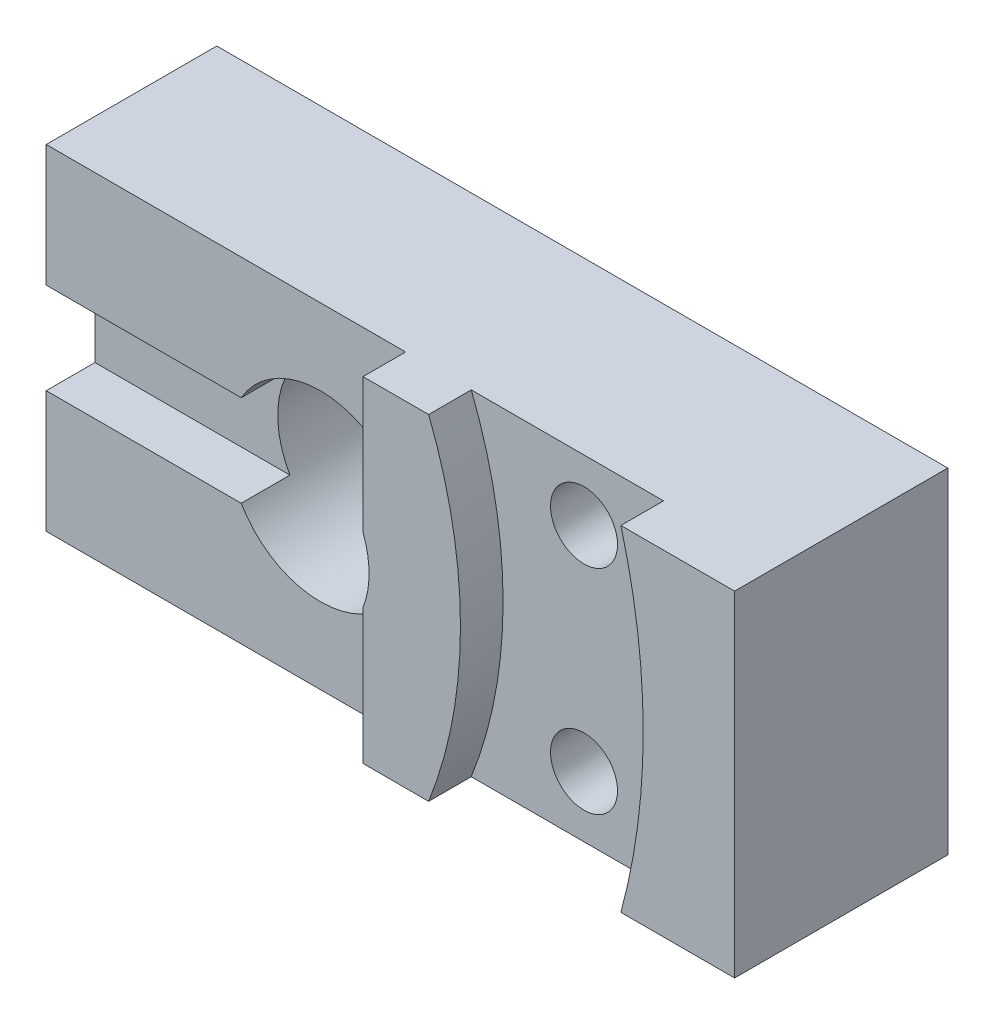
ISO-10303-21;
HEADER;
FILE_DESCRIPTION(('STEP AP214'),'2;1');
FILE_NAME('part.step','',(''),(''),'','','');
FILE_SCHEMA(('AUTOMOTIVE_DESIGN { 1 0 10303 214 1 1 1 1 }'));
ENDSEC;
DATA;
#1=APPLICATION_CONTEXT('core data for automotive mechanical design processes');
#2=APPLICATION_PROTOCOL_DEFINITION('international standard','automotive_design',2000,#1);
#3=PRODUCT_CONTEXT('',#1,'mechanical');
#4=PRODUCT('Part','Part','',(#3));
#5=PRODUCT_RELATED_PRODUCT_CATEGORY('part','',(#4));
#6=PRODUCT_DEFINITION_FORMATION('','',#4);
#7=PRODUCT_DEFINITION_CONTEXT('part definition',#1,'design');
#8=PRODUCT_DEFINITION('design','',#6,#7);
#9=PRODUCT_DEFINITION_SHAPE('','',#8);
#10=(LENGTH_UNIT() NAMED_UNIT(*) SI_UNIT(.MILLI.,.METRE.));
#11=(NAMED_UNIT(*) PLANE_ANGLE_UNIT() SI_UNIT($,.RADIAN.));
#12=(NAMED_UNIT(*) SI_UNIT($,.STERADIAN.) SOLID_ANGLE_UNIT());
#13=UNCERTAINTY_MEASURE_WITH_UNIT(LENGTH_MEASURE(1.E-05),#10,'distance_accuracy_value','');
#14=(GEOMETRIC_REPRESENTATION_CONTEXT(3) GLOBAL_UNCERTAINTY_ASSIGNED_CONTEXT((#13)) GLOBAL_UNIT_ASSIGNED_CONTEXT((#10,
#11,#12)) REPRESENTATION_CONTEXT('',''));
#15=CARTESIAN_POINT('',(0.,0.,0.));
#16=DIRECTION('',(0.,0.,1.));
#17=DIRECTION('',(1.,0.,0.));
#18=AXIS2_PLACEMENT_3D('',#15,#16,#17);
#19=CARTESIAN_POINT('',(0.,0.,28.));
#20=DIRECTION('',(0.,0.,-1.));
#21=DIRECTION('',(-1.,0.,0.));
#22=AXIS2_PLACEMENT_3D('',#19,#20,#21);
#23=PLANE('',#22);
#24=DIRECTION('',(0.,1.,0.));
#25=VECTOR('',#24,1.);
#26=CARTESIAN_POINT('',(-1.,0.,28.));
#27=LINE('',#26,#25);
#28=CARTESIAN_POINT('',(-1.,0.,28.));
#29=VERTEX_POINT('',#28);
#30=CARTESIAN_POINT('',(-1.,20.,28.));
#31=VERTEX_POINT('',#30);
#32=EDGE_CURVE('E204',#29,#31,#27,.T.);
#33=ORIENTED_EDGE('',*,*,#32,.T.);
#34=DIRECTION('',(-1.,0.,0.));
#35=VECTOR('',#34,1.);
#36=CARTESIAN_POINT('',(-1.,20.,28.));
#37=LINE('',#36,#35);
#38=CARTESIAN_POINT('',(-2.00961894323342,20.,28.));
#39=VERTEX_POINT('',#38);
#40=EDGE_CURVE('E328',#31,#39,#37,.T.);
#41=ORIENTED_EDGE('',*,*,#40,.T.);
#42=CARTESIAN_POINT('',(-15.,27.5,28.));
#43=DIRECTION('',(0.,0.,-1.));
#44=DIRECTION('',(-1.,0.,0.));
#45=AXIS2_PLACEMENT_3D('',#42,#43,#44);
#46=CIRCLE('',#45,15.);
#47=CARTESIAN_POINT('',(-27.9903810567666,20.,28.));
#48=VERTEX_POINT('',#47);
#49=EDGE_CURVE('E296',#39,#48,#46,.T.);
#50=ORIENTED_EDGE('',*,*,#49,.T.);
#51=DIRECTION('',(-1.,0.,0.));
#52=VECTOR('',#51,1.);
#53=CARTESIAN_POINT('',(0.,20.,28.));
#54=LINE('',#53,#52);
#55=CARTESIAN_POINT('',(-60.,20.,28.));
#56=VERTEX_POINT('',#55);
#57=EDGE_CURVE('E305',#48,#56,#54,.T.);
#58=ORIENTED_EDGE('',*,*,#57,.T.);
#59=DIRECTION('',(0.,-1.,0.));
#60=VECTOR('',#59,1.);
#61=CARTESIAN_POINT('',(-60.,0.,28.));
#62=LINE('',#61,#60);
#63=CARTESIAN_POINT('',(-60.,0.,28.));
#64=VERTEX_POINT('',#63);
#65=EDGE_CURVE('E217',#56,#64,#62,.T.);
#66=ORIENTED_EDGE('',*,*,#65,.T.);
#67=DIRECTION('',(1.,0.,0.));
#68=VECTOR('',#67,1.);
#69=CARTESIAN_POINT('',(-60.,0.,28.));
#70=LINE('',#69,#68);
#71=EDGE_CURVE('E202',#64,#29,#70,.T.);
#72=ORIENTED_EDGE('',*,*,#71,.T.);
#73=EDGE_LOOP('',(#33,#41,#50,#58,#66,#72));
#74=FACE_BOUND('',#73,.T.);
#75=ADVANCED_FACE('F39',(#74),#23,.F.);
#76=CARTESIAN_POINT('',(0.,0.,35.));
#77=DIRECTION('',(0.,0.,-1.));
#78=DIRECTION('',(-1.,0.,0.));
#79=AXIS2_PLACEMENT_3D('',#76,#77,#78);
#80=PLANE('',#79);
#81=DIRECTION('',(-1.,0.,0.));
#82=VECTOR('',#81,1.);
#83=CARTESIAN_POINT('',(-60.,55.,35.));
#84=LINE('',#83,#82);
#85=CARTESIAN_POINT('',(9.77642868476431,55.,35.));
#86=VERTEX_POINT('',#85);
#87=CARTESIAN_POINT('',(-1.,55.,35.));
#88=VERTEX_POINT('',#87);
#89=EDGE_CURVE('E269',#86,#88,#84,.T.);
#90=ORIENTED_EDGE('',*,*,#89,.T.);
#91=DIRECTION('',(0.,1.,0.));
#92=VECTOR('',#91,1.);
#93=CARTESIAN_POINT('',(-1.,0.,35.));
#94=LINE('',#93,#92);
#95=CARTESIAN_POINT('',(-1.,32.8851648071345,35.));
#96=VERTEX_POINT('',#95);
#97=EDGE_CURVE('E218',#96,#88,#94,.T.);
#98=ORIENTED_EDGE('',*,*,#97,.F.);
#99=CARTESIAN_POINT('',(-15.,27.5,35.));
#100=DIRECTION('',(0.,0.,1.));
#101=DIRECTION('',(1.,0.,0.));
#102=AXIS2_PLACEMENT_3D('',#99,#100,#101);
#103=CIRCLE('',#102,15.);
#104=CARTESIAN_POINT('',(-1.,22.1148351928655,35.));
#105=VERTEX_POINT('',#104);
#106=EDGE_CURVE('E259',#105,#96,#103,.T.);
#107=ORIENTED_EDGE('',*,*,#106,.F.);
#108=CARTESIAN_POINT('',(-1.,0.,35.));
#109=VERTEX_POINT('',#108);
#110=EDGE_CURVE('E216',#109,#105,#94,.T.);
#111=ORIENTED_EDGE('',*,*,#110,.F.);
#112=DIRECTION('',(1.,0.,0.));
#113=VECTOR('',#112,1.);
#114=CARTESIAN_POINT('',(-60.,0.,35.));
#115=LINE('',#114,#113);
#116=CARTESIAN_POINT('',(9.7764286847643,0.,35.));
#117=VERTEX_POINT('',#116);
#118=EDGE_CURVE('E264',#109,#117,#115,.T.);
#119=ORIENTED_EDGE('',*,*,#118,.T.);
#120=CARTESIAN_POINT('',(-60.,27.5,35.));
#121=DIRECTION('',(0.,0.,-1.));
#122=DIRECTION('',(1.,0.,0.));
#123=AXIS2_PLACEMENT_3D('',#120,#121,#122);
#124=CIRCLE('',#123,75.);
#125=EDGE_CURVE('E222',#86,#117,#124,.T.);
#126=ORIENTED_EDGE('',*,*,#125,.F.);
#127=EDGE_LOOP('',(#90,#98,#107,#111,#119,#126));
#128=FACE_BOUND('',#127,.T.);
#129=ADVANCED_FACE('F383',(#128),#80,.F.);
#130=CARTESIAN_POINT('',(28.2822179150479,45.,35.));
#131=DIRECTION('',(0.,0.,-1.));
#132=DIRECTION('',(-1.,0.,0.));
#133=AXIS2_PLACEMENT_3D('',#130,#131,#132);
#134=CYLINDRICAL_SURFACE('',#133,5.5);
#135=CARTESIAN_POINT('',(28.2822179150479,45.,0.));
#136=DIRECTION('',(0.,0.,1.));
#137=DIRECTION('',(1.,0.,0.));
#138=AXIS2_PLACEMENT_3D('',#135,#136,#137);
#139=CIRCLE('',#138,5.5);
#140=CARTESIAN_POINT('',(33.7822179150479,45.,0.));
#141=VERTEX_POINT('',#140);
#142=EDGE_CURVE('E254',#141,#141,#139,.T.);
#143=ORIENTED_EDGE('',*,*,#142,.F.);
#144=EDGE_LOOP('',(#143));
#145=FACE_BOUND('',#144,.T.);
#146=CARTESIAN_POINT('',(28.2822179150479,45.,28.));
#147=DIRECTION('',(0.,0.,1.));
#148=DIRECTION('',(1.,0.,0.));
#149=AXIS2_PLACEMENT_3D('',#146,#147,#148);
#150=CIRCLE('',#149,5.5);
#151=CARTESIAN_POINT('',(33.7822179150479,45.,28.));
#152=VERTEX_POINT('',#151);
#153=EDGE_CURVE('E249',#152,#152,#150,.T.);
#154=ORIENTED_EDGE('',*,*,#153,.T.);
#155=EDGE_LOOP('',(#154));
#156=FACE_BOUND('',#155,.T.);
#157=ADVANCED_FACE('F420',(#145,#156),#134,.F.);
#158=CARTESIAN_POINT('',(28.2822179150479,10.,35.));
#159=DIRECTION('',(0.,0.,-1.));
#160=DIRECTION('',(-1.,0.,0.));
#161=AXIS2_PLACEMENT_3D('',#158,#159,#160);
#162=CYLINDRICAL_SURFACE('',#161,5.5);
#163=CARTESIAN_POINT('',(28.2822179150479,10.,0.));
#164=DIRECTION('',(0.,0.,1.));
#165=DIRECTION('',(1.,0.,0.));
#166=AXIS2_PLACEMENT_3D('',#163,#164,#165);
#167=CIRCLE('',#166,5.5);
#168=CARTESIAN_POINT('',(33.7822179150479,10.,0.));
#169=VERTEX_POINT('',#168);
#170=EDGE_CURVE('E252',#169,#169,#167,.T.);
#171=ORIENTED_EDGE('',*,*,#170,.F.);
#172=EDGE_LOOP('',(#171));
#173=FACE_BOUND('',#172,.T.);
#174=CARTESIAN_POINT('',(28.2822179150479,10.,28.));
#175=DIRECTION('',(0.,0.,1.));
#176=DIRECTION('',(1.,0.,0.));
#177=AXIS2_PLACEMENT_3D('',#174,#175,#176);
#178=CIRCLE('',#177,5.5);
#179=CARTESIAN_POINT('',(33.7822179150479,10.,28.));
#180=VERTEX_POINT('',#179);
#181=EDGE_CURVE('E241',#180,#180,#178,.T.);
#182=ORIENTED_EDGE('',*,*,#181,.T.);
#183=EDGE_LOOP('',(#182));
#184=FACE_BOUND('',#183,.T.);
#185=ADVANCED_FACE('F437',(#173,#184),#162,.F.);
#186=CARTESIAN_POINT('',(60.,55.,35.));
#187=VERTEX_POINT('',#186);
#188=CARTESIAN_POINT('',(41.3348409975562,55.,35.));
#189=VERTEX_POINT('',#188);
#190=EDGE_CURVE('E271',#187,#189,#84,.T.);
#191=ORIENTED_EDGE('',*,*,#190,.T.);
#192=CARTESIAN_POINT('',(-60.,27.5,35.));
#193=DIRECTION('',(0.,0.,1.));
#194=DIRECTION('',(1.,0.,0.));
#195=AXIS2_PLACEMENT_3D('',#192,#193,#194);
#196=CIRCLE('',#195,105.);
#197=CARTESIAN_POINT('',(41.3348409975562,0.,35.));
#198=VERTEX_POINT('',#197);
#199=EDGE_CURVE('E230',#198,#189,#196,.T.);
#200=ORIENTED_EDGE('',*,*,#199,.F.);
#201=CARTESIAN_POINT('',(60.,0.,35.));
#202=VERTEX_POINT('',#201);
#203=EDGE_CURVE('E268',#198,#202,#115,.T.);
#204=ORIENTED_EDGE('',*,*,#203,.T.);
#205=DIRECTION('',(0.,1.,0.));
#206=VECTOR('',#205,1.);
#207=CARTESIAN_POINT('',(60.,0.,35.));
#208=LINE('',#207,#206);
#209=EDGE_CURVE('E270',#202,#187,#208,.T.);
#210=ORIENTED_EDGE('',*,*,#209,.T.);
#211=EDGE_LOOP('',(#191,#200,#204,#210));
#212=FACE_BOUND('',#211,.T.);
#213=ADVANCED_FACE('F370',(#212),#80,.F.);
#214=CARTESIAN_POINT('',(0.,0.,0.));
#215=DIRECTION('',(0.,0.,-1.));
#216=DIRECTION('',(-1.,0.,0.));
#217=AXIS2_PLACEMENT_3D('',#214,#215,#216);
#218=PLANE('',#217);
#219=ORIENTED_EDGE('',*,*,#142,.T.);
#220=EDGE_LOOP('',(#219));
#221=FACE_BOUND('',#220,.T.);
#222=DIRECTION('',(0.,-1.,0.));
#223=VECTOR('',#222,1.);
#224=CARTESIAN_POINT('',(-60.,0.,0.));
#225=LINE('',#224,#223);
#226=CARTESIAN_POINT('',(-60.,55.,0.));
#227=VERTEX_POINT('',#226);
#228=CARTESIAN_POINT('',(-60.,0.,0.));
#229=VERTEX_POINT('',#228);
#230=EDGE_CURVE('E265',#227,#229,#225,.T.);
#231=ORIENTED_EDGE('',*,*,#230,.F.);
#232=DIRECTION('',(-1.,0.,0.));
#233=VECTOR('',#232,1.);
#234=CARTESIAN_POINT('',(-60.,55.,0.));
#235=LINE('',#234,#233);
#236=CARTESIAN_POINT('',(60.,55.,0.));
#237=VERTEX_POINT('',#236);
#238=EDGE_CURVE('E281',#237,#227,#235,.T.);
#239=ORIENTED_EDGE('',*,*,#238,.F.);
#240=DIRECTION('',(0.,1.,0.));
#241=VECTOR('',#240,1.);
#242=CARTESIAN_POINT('',(60.,0.,0.));
#243=LINE('',#242,#241);
#244=CARTESIAN_POINT('',(60.,0.,0.));
#245=VERTEX_POINT('',#244);
#246=EDGE_CURVE('E276',#245,#237,#243,.T.);
#247=ORIENTED_EDGE('',*,*,#246,.F.);
#248=DIRECTION('',(1.,0.,0.));
#249=VECTOR('',#248,1.);
#250=CARTESIAN_POINT('',(-60.,0.,0.));
#251=LINE('',#250,#249);
#252=EDGE_CURVE('E280',#229,#245,#251,.T.);
#253=ORIENTED_EDGE('',*,*,#252,.F.);
#254=EDGE_LOOP('',(#231,#239,#247,#253));
#255=FACE_BOUND('',#254,.T.);
#256=CARTESIAN_POINT('',(-15.,27.5,0.));
#257=DIRECTION('',(0.,0.,1.));
#258=DIRECTION('',(1.,0.,0.));
#259=AXIS2_PLACEMENT_3D('',#256,#257,#258);
#260=CIRCLE('',#259,15.);
#261=CARTESIAN_POINT('',(0.,27.5,0.));
#262=VERTEX_POINT('',#261);
#263=EDGE_CURVE('E256',#262,#262,#260,.T.);
#264=ORIENTED_EDGE('',*,*,#263,.T.);
#265=EDGE_LOOP('',(#264));
#266=FACE_BOUND('',#265,.T.);
#267=ORIENTED_EDGE('',*,*,#170,.T.);
#268=EDGE_LOOP('',(#267));
#269=FACE_BOUND('',#268,.T.);
#270=ADVANCED_FACE('F358',(#221,#255,#266,#269),#218,.T.);
#271=CARTESIAN_POINT('',(-60.,0.,35.));
#272=DIRECTION('',(1.,0.,0.));
#273=DIRECTION('',(0.,0.,-1.));
#274=AXIS2_PLACEMENT_3D('',#271,#272,#273);
#275=PLANE('',#274);
#276=ORIENTED_EDGE('',*,*,#65,.F.);
#277=DIRECTION('',(0.,0.,1.));
#278=VECTOR('',#277,1.);
#279=CARTESIAN_POINT('',(-60.,20.,28.));
#280=LINE('',#279,#278);
#281=CARTESIAN_POINT('',(-60.,20.,20.));
#282=VERTEX_POINT('',#281);
#283=EDGE_CURVE('E187',#282,#56,#280,.T.);
#284=ORIENTED_EDGE('',*,*,#283,.F.);
#285=DIRECTION('',(0.,-1.,0.));
#286=VECTOR('',#285,1.);
#287=CARTESIAN_POINT('',(-60.,20.,20.));
#288=LINE('',#287,#286);
#289=CARTESIAN_POINT('',(-60.,35.,20.));
#290=VERTEX_POINT('',#289);
#291=EDGE_CURVE('E324',#290,#282,#288,.T.);
#292=ORIENTED_EDGE('',*,*,#291,.F.);
#293=DIRECTION('',(0.,0.,-1.));
#294=VECTOR('',#293,1.);
#295=CARTESIAN_POINT('',(-60.,35.,28.));
#296=LINE('',#295,#294);
#297=CARTESIAN_POINT('',(-60.,35.,28.));
#298=VERTEX_POINT('',#297);
#299=EDGE_CURVE('E325',#298,#290,#296,.T.);
#300=ORIENTED_EDGE('',*,*,#299,.F.);
#301=CARTESIAN_POINT('',(-60.,55.,28.));
#302=VERTEX_POINT('',#301);
#303=EDGE_CURVE('E209',#302,#298,#62,.T.);
#304=ORIENTED_EDGE('',*,*,#303,.F.);
#305=DIRECTION('',(0.,0.,-1.));
#306=VECTOR('',#305,1.);
#307=CARTESIAN_POINT('',(-60.,55.,35.));
#308=LINE('',#307,#306);
#309=EDGE_CURVE('E273',#302,#227,#308,.T.);
#310=ORIENTED_EDGE('',*,*,#309,.T.);
#311=ORIENTED_EDGE('',*,*,#230,.T.);
#312=DIRECTION('',(0.,0.,-1.));
#313=VECTOR('',#312,1.);
#314=CARTESIAN_POINT('',(-60.,0.,35.));
#315=LINE('',#314,#313);
#316=EDGE_CURVE('E292',#64,#229,#315,.T.);
#317=ORIENTED_EDGE('',*,*,#316,.F.);
#318=EDGE_LOOP('',(#276,#284,#292,#300,#304,#310,#311,#317));
#319=FACE_BOUND('',#318,.T.);
#320=ADVANCED_FACE('F41',(#319),#275,.F.);
#321=CARTESIAN_POINT('',(-60.,0.,35.));
#322=DIRECTION('',(0.,1.,0.));
#323=DIRECTION('',(-1.,0.,0.));
#324=AXIS2_PLACEMENT_3D('',#321,#322,#323);
#325=PLANE('',#324);
#326=ORIENTED_EDGE('',*,*,#118,.F.);
#327=DIRECTION('',(0.,0.,1.));
#328=VECTOR('',#327,1.);
#329=CARTESIAN_POINT('',(-1.,0.,28.));
#330=LINE('',#329,#328);
#331=EDGE_CURVE('E214',#29,#109,#330,.T.);
#332=ORIENTED_EDGE('',*,*,#331,.F.);
#333=ORIENTED_EDGE('',*,*,#71,.F.);
#334=ORIENTED_EDGE('',*,*,#316,.T.);
#335=ORIENTED_EDGE('',*,*,#252,.T.);
#336=DIRECTION('',(0.,0.,-1.));
#337=VECTOR('',#336,1.);
#338=CARTESIAN_POINT('',(60.,0.,35.));
#339=LINE('',#338,#337);
#340=EDGE_CURVE('E286',#202,#245,#339,.T.);
#341=ORIENTED_EDGE('',*,*,#340,.F.);
#342=ORIENTED_EDGE('',*,*,#203,.F.);
#343=DIRECTION('',(0.,0.,1.));
#344=VECTOR('',#343,1.);
#345=CARTESIAN_POINT('',(41.3348409975562,0.,28.));
#346=LINE('',#345,#344);
#347=CARTESIAN_POINT('',(41.3348409975562,0.,28.));
#348=VERTEX_POINT('',#347);
#349=EDGE_CURVE('E244',#348,#198,#346,.T.);
#350=ORIENTED_EDGE('',*,*,#349,.F.);
#351=DIRECTION('',(1.,0.,0.));
#352=VECTOR('',#351,1.);
#353=CARTESIAN_POINT('',(9.7764286847643,0.,28.));
#354=LINE('',#353,#352);
#355=CARTESIAN_POINT('',(9.7764286847643,0.,28.));
#356=VERTEX_POINT('',#355);
#357=EDGE_CURVE('E226',#356,#348,#354,.T.);
#358=ORIENTED_EDGE('',*,*,#357,.F.);
#359=DIRECTION('',(0.,0.,1.));
#360=VECTOR('',#359,1.);
#361=CARTESIAN_POINT('',(9.7764286847643,0.,28.));
#362=LINE('',#361,#360);
#363=EDGE_CURVE('E232',#356,#117,#362,.T.);
#364=ORIENTED_EDGE('',*,*,#363,.T.);
#365=EDGE_LOOP('',(#326,#332,#333,#334,#335,#341,#342,#350,#358,#364));
#366=FACE_BOUND('',#365,.T.);
#367=ADVANCED_FACE('F348',(#366),#325,.F.);
#368=CARTESIAN_POINT('',(60.,0.,35.));
#369=DIRECTION('',(-1.,0.,0.));
#370=DIRECTION('',(0.,-1.,0.));
#371=AXIS2_PLACEMENT_3D('',#368,#369,#370);
#372=PLANE('',#371);
#373=ORIENTED_EDGE('',*,*,#246,.T.);
#374=DIRECTION('',(0.,0.,-1.));
#375=VECTOR('',#374,1.);
#376=CARTESIAN_POINT('',(60.,55.,35.));
#377=LINE('',#376,#375);
#378=EDGE_CURVE('E284',#187,#237,#377,.T.);
#379=ORIENTED_EDGE('',*,*,#378,.F.);
#380=ORIENTED_EDGE('',*,*,#209,.F.);
#381=ORIENTED_EDGE('',*,*,#340,.T.);
#382=EDGE_LOOP('',(#373,#379,#380,#381));
#383=FACE_BOUND('',#382,.T.);
#384=ADVANCED_FACE('F361',(#383),#372,.F.);
#385=CARTESIAN_POINT('',(-60.,55.,35.));
#386=DIRECTION('',(0.,-1.,0.));
#387=DIRECTION('',(1.,0.,0.));
#388=AXIS2_PLACEMENT_3D('',#385,#386,#387);
#389=PLANE('',#388);
#390=DIRECTION('',(-1.,0.,0.));
#391=VECTOR('',#390,1.);
#392=CARTESIAN_POINT('',(-60.,55.,28.));
#393=LINE('',#392,#391);
#394=CARTESIAN_POINT('',(-1.,55.,28.));
#395=VERTEX_POINT('',#394);
#396=EDGE_CURVE('E208',#395,#302,#393,.T.);
#397=ORIENTED_EDGE('',*,*,#396,.F.);
#398=DIRECTION('',(0.,0.,1.));
#399=VECTOR('',#398,1.);
#400=CARTESIAN_POINT('',(-1.,55.,28.));
#401=LINE('',#400,#399);
#402=EDGE_CURVE('E205',#395,#88,#401,.T.);
#403=ORIENTED_EDGE('',*,*,#402,.T.);
#404=ORIENTED_EDGE('',*,*,#89,.F.);
#405=DIRECTION('',(0.,0.,1.));
#406=VECTOR('',#405,1.);
#407=CARTESIAN_POINT('',(9.77642868476431,55.,28.));
#408=LINE('',#407,#406);
#409=CARTESIAN_POINT('',(9.77642868476431,55.,28.));
#410=VERTEX_POINT('',#409);
#411=EDGE_CURVE('E239',#410,#86,#408,.T.);
#412=ORIENTED_EDGE('',*,*,#411,.F.);
#413=DIRECTION('',(-1.,0.,0.));
#414=VECTOR('',#413,1.);
#415=CARTESIAN_POINT('',(9.77642868476431,55.,28.));
#416=LINE('',#415,#414);
#417=CARTESIAN_POINT('',(41.3348409975562,55.,28.));
#418=VERTEX_POINT('',#417);
#419=EDGE_CURVE('E235',#418,#410,#416,.T.);
#420=ORIENTED_EDGE('',*,*,#419,.F.);
#421=DIRECTION('',(0.,0.,1.));
#422=VECTOR('',#421,1.);
#423=CARTESIAN_POINT('',(41.3348409975562,55.,28.));
#424=LINE('',#423,#422);
#425=EDGE_CURVE('E245',#418,#189,#424,.T.);
#426=ORIENTED_EDGE('',*,*,#425,.T.);
#427=ORIENTED_EDGE('',*,*,#190,.F.);
#428=ORIENTED_EDGE('',*,*,#378,.T.);
#429=ORIENTED_EDGE('',*,*,#238,.T.);
#430=ORIENTED_EDGE('',*,*,#309,.F.);
#431=EDGE_LOOP('',(#397,#403,#404,#412,#420,#426,#427,#428,#429,#430));
#432=FACE_BOUND('',#431,.T.);
#433=ADVANCED_FACE('F446',(#432),#389,.F.);
#434=CARTESIAN_POINT('',(-15.,27.5,35.));
#435=DIRECTION('',(0.,0.,-1.));
#436=DIRECTION('',(-1.,0.,0.));
#437=AXIS2_PLACEMENT_3D('',#434,#435,#436);
#438=CYLINDRICAL_SURFACE('',#437,15.);
#439=DIRECTION('',(0.,0.,-1.));
#440=VECTOR('',#439,1.);
#441=CARTESIAN_POINT('',(-27.9903810567666,20.,35.));
#442=LINE('',#441,#440);
#443=CARTESIAN_POINT('',(-27.9903810567666,20.,20.));
#444=VERTEX_POINT('',#443);
#445=EDGE_CURVE('E343',#48,#444,#442,.T.);
#446=ORIENTED_EDGE('',*,*,#445,.F.);
#447=ORIENTED_EDGE('',*,*,#49,.F.);
#448=DIRECTION('',(0.,0.,-1.));
#449=VECTOR('',#448,1.);
#450=CARTESIAN_POINT('',(-2.00961894323342,20.,35.));
#451=LINE('',#450,#449);
#452=CARTESIAN_POINT('',(-2.00961894323342,20.,20.));
#453=VERTEX_POINT('',#452);
#454=EDGE_CURVE('E338',#453,#39,#451,.F.);
#455=ORIENTED_EDGE('',*,*,#454,.F.);
#456=CARTESIAN_POINT('',(-15.,27.5,20.));
#457=DIRECTION('',(0.,0.,-1.));
#458=DIRECTION('',(-1.,0.,0.));
#459=AXIS2_PLACEMENT_3D('',#456,#457,#458);
#460=CIRCLE('',#459,15.);
#461=CARTESIAN_POINT('',(-1.,22.1148351928655,20.));
#462=VERTEX_POINT('',#461);
#463=EDGE_CURVE('E43',#462,#453,#460,.T.);
#464=ORIENTED_EDGE('',*,*,#463,.F.);
#465=DIRECTION('',(0.,0.,-1.));
#466=VECTOR('',#465,1.);
#467=CARTESIAN_POINT('',(-1.,22.1148351928655,35.));
#468=LINE('',#467,#466);
#469=EDGE_CURVE('E298',#105,#462,#468,.T.);
#470=ORIENTED_EDGE('',*,*,#469,.F.);
#471=ORIENTED_EDGE('',*,*,#106,.T.);
#472=DIRECTION('',(0.,0.,-1.));
#473=VECTOR('',#472,1.);
#474=CARTESIAN_POINT('',(-1.,32.8851648071345,35.));
#475=LINE('',#474,#473);
#476=CARTESIAN_POINT('',(-1.,32.8851648071345,20.));
#477=VERTEX_POINT('',#476);
#478=EDGE_CURVE('E300',#477,#96,#475,.F.);
#479=ORIENTED_EDGE('',*,*,#478,.F.);
#480=CARTESIAN_POINT('',(-2.00961894323342,35.,20.));
#481=VERTEX_POINT('',#480);
#482=EDGE_CURVE('E48',#481,#477,#460,.T.);
#483=ORIENTED_EDGE('',*,*,#482,.F.);
#484=DIRECTION('',(0.,0.,-1.));
#485=VECTOR('',#484,1.);
#486=CARTESIAN_POINT('',(-2.00961894323342,35.,35.));
#487=LINE('',#486,#485);
#488=CARTESIAN_POINT('',(-2.00961894323342,35.,28.));
#489=VERTEX_POINT('',#488);
#490=EDGE_CURVE('E340',#489,#481,#487,.T.);
#491=ORIENTED_EDGE('',*,*,#490,.F.);
#492=CARTESIAN_POINT('',(-27.9903810567666,35.,28.));
#493=VERTEX_POINT('',#492);
#494=EDGE_CURVE('E197',#493,#489,#46,.T.);
#495=ORIENTED_EDGE('',*,*,#494,.F.);
#496=DIRECTION('',(0.,0.,-1.));
#497=VECTOR('',#496,1.);
#498=CARTESIAN_POINT('',(-27.9903810567666,35.,35.));
#499=LINE('',#498,#497);
#500=CARTESIAN_POINT('',(-27.9903810567666,35.,20.));
#501=VERTEX_POINT('',#500);
#502=EDGE_CURVE('E62',#501,#493,#499,.F.);
#503=ORIENTED_EDGE('',*,*,#502,.F.);
#504=EDGE_CURVE('E11',#444,#501,#460,.T.);
#505=ORIENTED_EDGE('',*,*,#504,.F.);
#506=EDGE_LOOP('',(#446,#447,#455,#464,#470,#471,#479,#483,#491,#495,#503,#505));
#507=FACE_BOUND('',#506,.T.);
#508=ORIENTED_EDGE('',*,*,#263,.F.);
#509=EDGE_LOOP('',(#508));
#510=FACE_BOUND('',#509,.T.);
#511=ADVANCED_FACE('F388',(#507,#510),#438,.F.);
#512=CARTESIAN_POINT('',(-60.,27.5,28.));
#513=DIRECTION('',(0.,0.,1.));
#514=DIRECTION('',(1.,0.,0.));
#515=AXIS2_PLACEMENT_3D('',#512,#513,#514);
#516=CYLINDRICAL_SURFACE('',#515,75.);
#517=ORIENTED_EDGE('',*,*,#125,.T.);
#518=ORIENTED_EDGE('',*,*,#363,.F.);
#519=CARTESIAN_POINT('',(-60.,27.5,28.));
#520=DIRECTION('',(0.,0.,-1.));
#521=DIRECTION('',(1.,0.,0.));
#522=AXIS2_PLACEMENT_3D('',#519,#520,#521);
#523=CIRCLE('',#522,75.);
#524=EDGE_CURVE('E224',#410,#356,#523,.T.);
#525=ORIENTED_EDGE('',*,*,#524,.F.);
#526=ORIENTED_EDGE('',*,*,#411,.T.);
#527=EDGE_LOOP('',(#517,#518,#525,#526));
#528=FACE_BOUND('',#527,.T.);
#529=ADVANCED_FACE('F377',(#528),#516,.T.);
#530=CARTESIAN_POINT('',(-60.,27.5,28.));
#531=DIRECTION('',(0.,0.,1.));
#532=DIRECTION('',(1.,0.,0.));
#533=AXIS2_PLACEMENT_3D('',#530,#531,#532);
#534=CYLINDRICAL_SURFACE('',#533,105.);
#535=ORIENTED_EDGE('',*,*,#199,.T.);
#536=ORIENTED_EDGE('',*,*,#425,.F.);
#537=CARTESIAN_POINT('',(-60.,27.5,28.));
#538=DIRECTION('',(0.,0.,1.));
#539=DIRECTION('',(1.,0.,0.));
#540=AXIS2_PLACEMENT_3D('',#537,#538,#539);
#541=CIRCLE('',#540,105.);
#542=EDGE_CURVE('E229',#348,#418,#541,.T.);
#543=ORIENTED_EDGE('',*,*,#542,.F.);
#544=ORIENTED_EDGE('',*,*,#349,.T.);
#545=EDGE_LOOP('',(#535,#536,#543,#544));
#546=FACE_BOUND('',#545,.T.);
#547=ADVANCED_FACE('F375',(#546),#534,.F.);
#548=CARTESIAN_POINT('',(-60.,27.5,28.));
#549=DIRECTION('',(0.,0.,1.));
#550=DIRECTION('',(1.,0.,0.));
#551=AXIS2_PLACEMENT_3D('',#548,#549,#550);
#552=PLANE('',#551);
#553=ORIENTED_EDGE('',*,*,#153,.F.);
#554=EDGE_LOOP('',(#553));
#555=FACE_BOUND('',#554,.T.);
#556=ORIENTED_EDGE('',*,*,#181,.F.);
#557=EDGE_LOOP('',(#556));
#558=FACE_BOUND('',#557,.T.);
#559=ORIENTED_EDGE('',*,*,#524,.T.);
#560=ORIENTED_EDGE('',*,*,#357,.T.);
#561=ORIENTED_EDGE('',*,*,#542,.T.);
#562=ORIENTED_EDGE('',*,*,#419,.T.);
#563=EDGE_LOOP('',(#559,#560,#561,#562));
#564=FACE_BOUND('',#563,.T.);
#565=ADVANCED_FACE('F376',(#555,#558,#564),#552,.T.);
#566=CARTESIAN_POINT('',(-1.,0.,28.));
#567=DIRECTION('',(1.,0.,0.));
#568=DIRECTION('',(0.,0.,-1.));
#569=AXIS2_PLACEMENT_3D('',#566,#567,#568);
#570=PLANE('',#569);
#571=ORIENTED_EDGE('',*,*,#469,.T.);
#572=DIRECTION('',(0.,-1.,0.));
#573=VECTOR('',#572,1.);
#574=CARTESIAN_POINT('',(-1.,20.,20.));
#575=LINE('',#574,#573);
#576=CARTESIAN_POINT('',(-1.,20.,20.));
#577=VERTEX_POINT('',#576);
#578=EDGE_CURVE('E190',#462,#577,#575,.T.);
#579=ORIENTED_EDGE('',*,*,#578,.T.);
#580=DIRECTION('',(0.,0.,1.));
#581=VECTOR('',#580,1.);
#582=CARTESIAN_POINT('',(-1.,20.,28.));
#583=LINE('',#582,#581);
#584=EDGE_CURVE('E54',#577,#31,#583,.T.);
#585=ORIENTED_EDGE('',*,*,#584,.T.);
#586=ORIENTED_EDGE('',*,*,#32,.F.);
#587=ORIENTED_EDGE('',*,*,#331,.T.);
#588=ORIENTED_EDGE('',*,*,#110,.T.);
#589=EDGE_LOOP('',(#571,#579,#585,#586,#587,#588));
#590=FACE_BOUND('',#589,.T.);
#591=ADVANCED_FACE('F389',(#590),#570,.F.);
#592=ORIENTED_EDGE('',*,*,#478,.T.);
#593=ORIENTED_EDGE('',*,*,#97,.T.);
#594=ORIENTED_EDGE('',*,*,#402,.F.);
#595=CARTESIAN_POINT('',(-1.,35.,28.));
#596=VERTEX_POINT('',#595);
#597=EDGE_CURVE('E194',#596,#395,#27,.T.);
#598=ORIENTED_EDGE('',*,*,#597,.F.);
#599=DIRECTION('',(0.,0.,-1.));
#600=VECTOR('',#599,1.);
#601=CARTESIAN_POINT('',(-1.,35.,28.));
#602=LINE('',#601,#600);
#603=CARTESIAN_POINT('',(-1.,35.,20.));
#604=VERTEX_POINT('',#603);
#605=EDGE_CURVE('E178',#596,#604,#602,.T.);
#606=ORIENTED_EDGE('',*,*,#605,.T.);
#607=EDGE_CURVE('E316',#604,#477,#575,.T.);
#608=ORIENTED_EDGE('',*,*,#607,.T.);
#609=EDGE_LOOP('',(#592,#593,#594,#598,#606,#608));
#610=FACE_BOUND('',#609,.T.);
#611=ADVANCED_FACE('F199',(#610),#570,.F.);
#612=ORIENTED_EDGE('',*,*,#303,.T.);
#613=DIRECTION('',(1.,0.,0.));
#614=VECTOR('',#613,1.);
#615=CARTESIAN_POINT('',(0.,35.,28.));
#616=LINE('',#615,#614);
#617=EDGE_CURVE('E303',#298,#493,#616,.T.);
#618=ORIENTED_EDGE('',*,*,#617,.T.);
#619=ORIENTED_EDGE('',*,*,#494,.T.);
#620=DIRECTION('',(-1.,0.,0.));
#621=VECTOR('',#620,1.);
#622=CARTESIAN_POINT('',(-1.,35.,28.));
#623=LINE('',#622,#621);
#624=EDGE_CURVE('E179',#596,#489,#623,.T.);
#625=ORIENTED_EDGE('',*,*,#624,.F.);
#626=ORIENTED_EDGE('',*,*,#597,.T.);
#627=ORIENTED_EDGE('',*,*,#396,.T.);
#628=EDGE_LOOP('',(#612,#618,#619,#625,#626,#627));
#629=FACE_BOUND('',#628,.T.);
#630=ADVANCED_FACE('F191',(#629),#23,.F.);
#631=CARTESIAN_POINT('',(-1.,35.,28.));
#632=DIRECTION('',(0.,1.,0.));
#633=DIRECTION('',(0.,0.,1.));
#634=AXIS2_PLACEMENT_3D('',#631,#632,#633);
#635=PLANE('',#634);
#636=ORIENTED_EDGE('',*,*,#490,.T.);
#637=DIRECTION('',(-1.,0.,0.));
#638=VECTOR('',#637,1.);
#639=CARTESIAN_POINT('',(-1.,35.,20.));
#640=LINE('',#639,#638);
#641=EDGE_CURVE('E185',#604,#481,#640,.T.);
#642=ORIENTED_EDGE('',*,*,#641,.F.);
#643=ORIENTED_EDGE('',*,*,#605,.F.);
#644=ORIENTED_EDGE('',*,*,#624,.T.);
#645=EDGE_LOOP('',(#636,#642,#643,#644));
#646=FACE_BOUND('',#645,.T.);
#647=ADVANCED_FACE('F176',(#646),#635,.F.);
#648=CARTESIAN_POINT('',(-1.,20.,20.));
#649=DIRECTION('',(0.,0.,-1.));
#650=DIRECTION('',(-1.,0.,0.));
#651=AXIS2_PLACEMENT_3D('',#648,#649,#650);
#652=PLANE('',#651);
#653=ORIENTED_EDGE('',*,*,#482,.T.);
#654=ORIENTED_EDGE('',*,*,#607,.F.);
#655=ORIENTED_EDGE('',*,*,#641,.T.);
#656=EDGE_LOOP('',(#653,#654,#655));
#657=FACE_BOUND('',#656,.T.);
#658=ADVANCED_FACE('F312',(#657),#652,.F.);
#659=CARTESIAN_POINT('',(-1.,20.,28.));
#660=DIRECTION('',(0.,-1.,0.));
#661=DIRECTION('',(0.,0.,-1.));
#662=AXIS2_PLACEMENT_3D('',#659,#660,#661);
#663=PLANE('',#662);
#664=ORIENTED_EDGE('',*,*,#454,.T.);
#665=ORIENTED_EDGE('',*,*,#40,.F.);
#666=ORIENTED_EDGE('',*,*,#584,.F.);
#667=DIRECTION('',(-1.,0.,0.));
#668=VECTOR('',#667,1.);
#669=CARTESIAN_POINT('',(-1.,20.,20.));
#670=LINE('',#669,#668);
#671=EDGE_CURVE('E335',#577,#453,#670,.T.);
#672=ORIENTED_EDGE('',*,*,#671,.T.);
#673=EDGE_LOOP('',(#664,#665,#666,#672));
#674=FACE_BOUND('',#673,.T.);
#675=ADVANCED_FACE('F394',(#674),#663,.F.);
#676=ORIENTED_EDGE('',*,*,#463,.T.);
#677=ORIENTED_EDGE('',*,*,#671,.F.);
#678=ORIENTED_EDGE('',*,*,#578,.F.);
#679=EDGE_LOOP('',(#676,#677,#678));
#680=FACE_BOUND('',#679,.T.);
#681=ADVANCED_FACE('F398',(#680),#652,.F.);
#682=ORIENTED_EDGE('',*,*,#445,.T.);
#683=EDGE_CURVE('E331',#444,#282,#670,.T.);
#684=ORIENTED_EDGE('',*,*,#683,.T.);
#685=ORIENTED_EDGE('',*,*,#283,.T.);
#686=ORIENTED_EDGE('',*,*,#57,.F.);
#687=EDGE_LOOP('',(#682,#684,#685,#686));
#688=FACE_BOUND('',#687,.T.);
#689=ADVANCED_FACE('F396',(#688),#663,.F.);
#690=ORIENTED_EDGE('',*,*,#504,.T.);
#691=EDGE_CURVE('E196',#501,#290,#640,.T.);
#692=ORIENTED_EDGE('',*,*,#691,.T.);
#693=ORIENTED_EDGE('',*,*,#291,.T.);
#694=ORIENTED_EDGE('',*,*,#683,.F.);
#695=EDGE_LOOP('',(#690,#692,#693,#694));
#696=FACE_BOUND('',#695,.T.);
#697=ADVANCED_FACE('F397',(#696),#652,.F.);
#698=ORIENTED_EDGE('',*,*,#502,.T.);
#699=ORIENTED_EDGE('',*,*,#617,.F.);
#700=ORIENTED_EDGE('',*,*,#299,.T.);
#701=ORIENTED_EDGE('',*,*,#691,.F.);
#702=EDGE_LOOP('',(#698,#699,#700,#701));
#703=FACE_BOUND('',#702,.T.);
#704=ADVANCED_FACE('F408',(#703),#635,.F.);
#705=CLOSED_SHELL('',(#75,#129,#157,#185,#213,#270,#320,#367,#384,#433,#511,#529,#547,#565,#591,
#611,#630,#647,#658,#675,#681,#689,#697,#704));
#706=MANIFOLD_SOLID_BREP('B2',#705);
#707=ADVANCED_BREP_SHAPE_REPRESENTATION('',(#18,#706),#14);
#708=SHAPE_DEFINITION_REPRESENTATION(#9,#707);
ENDSEC;
END-ISO-10303-21;
